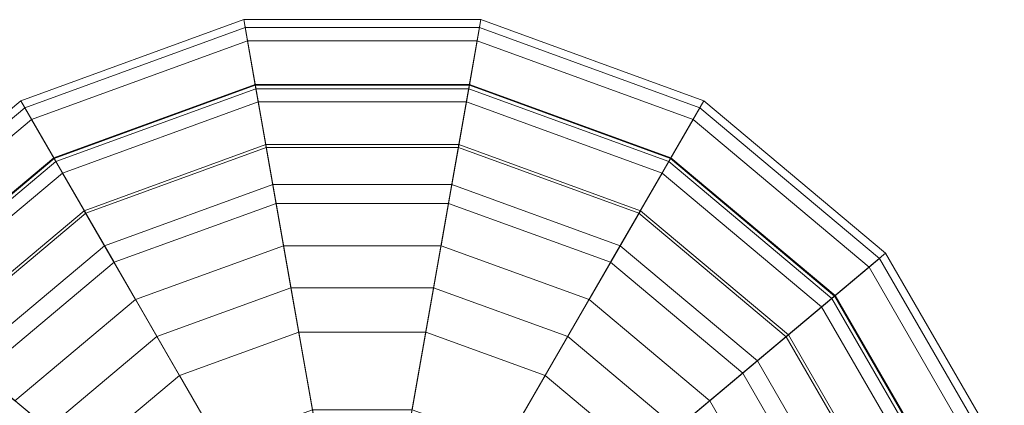
# Model space of a CAD drawing. Units: inches. Extents: x 375 to 1122, y 27 to 1069.
# Tile 23 of 155: x 718.584 to 720.536, y 273.809 to 274.574. Entities that reach past the tile are written whole.
import ezdxf

# ---------------------------------------------------------------- set-up
doc = ezdxf.new("R2010")
doc.units = ezdxf.units.IN
doc.layers.add('Furniture', color=30, linetype='Continuous', lineweight=18)

# ---------------------------------------------------------------- blocks, each defined once
blk = doc.blocks.new('A$C403C54AD')
for points in [[(1.816094, 0.886635, -0.028594), (1.814977, 0.889704, -0.031825), (1.804793, 0.883824, -0.031825), (1.806892, 0.881322, -0.028594)], [(1.814977, 0.889704, -0.031825), (1.826559, 0.857884, -0.028747), (1.826559, 0.857884, -0.028747), (1.804793, 0.883824, -0.031825)], [(1.816108, 0.886597, 0.131159), (1.815114, 0.889329, 0.117935), (1.805049, 0.883518, 0.117935), (1.806918, 0.881291, 0.131159)], [(1.815114, 0.889329, 0.117935), (1.815345, 0.888695, 0.089693), (1.805483, 0.883001, 0.089693), (1.805049, 0.883518, 0.117935)], [(1.815345, 0.888695, 0.089693), (1.817179, 0.883654, 0.071684), (1.808931, 0.878892, 0.071684), (1.805483, 0.883001, 0.089693)], [(1.821697, 0.871241, -0.02532), (1.816094, 0.886635, -0.028594), (1.806892, 0.881322, -0.028594), (1.817422, 0.868773, -0.02532)], [(1.817817, 0.881902, 0.140564), (1.816108, 0.886597, 0.131159), (1.806918, 0.881291, 0.131159), (1.81013, 0.877464, 0.140564)], [(1.816169, 0.886431, 0.117718), (1.81713, 0.88379, 0.130354), (1.808838, 0.879003, 0.130354), (1.807032, 0.881156, 0.117718)], [(1.816394, 0.885812, 0.090178), (1.816169, 0.886431, 0.117718), (1.807032, 0.881156, 0.117718), (1.807455, 0.880651, 0.090178)], [(1.818141, 0.881013, 0.073031), (1.816394, 0.885812, 0.090178), (1.807455, 0.880651, 0.090178), (1.810738, 0.876739, 0.073031)], [(1.806892, 0.881322, -0.028594), (1.804793, 0.883824, -0.031825), (1.797233, 0.874815, -0.031825), (1.800062, 0.873182, -0.028594)], [(1.804793, 0.883824, -0.031825), (1.826559, 0.857884, -0.028747), (1.826559, 0.857884, -0.028747), (1.797233, 0.874815, -0.031825)], [(1.806918, 0.881291, 0.131159), (1.805049, 0.883518, 0.117935), (1.797579, 0.874616, 0.117935), (1.800097, 0.873162, 0.131159)], [(1.805049, 0.883518, 0.117935), (1.805483, 0.883001, 0.089693), (1.798163, 0.874278, 0.089693), (1.797579, 0.874616, 0.117935)], [(1.81713, 0.88379, 0.130354), (1.81887, 0.879009, 0.140564), (1.812108, 0.875106, 0.140564), (1.808838, 0.879003, 0.130354)], [(1.817179, 0.883654, 0.071684), (1.819596, 0.877014, 0.061451), (1.813473, 0.873479, 0.061451), (1.808931, 0.878892, 0.071684)], [(1.805483, 0.883001, 0.089693), (1.808931, 0.878892, 0.071684), (1.802809, 0.871596, 0.071684), (1.798163, 0.874278, 0.089693)], [(1.81887, 0.879009, 0.140564), (1.817817, 0.881902, 0.140564), (1.81013, 0.877464, 0.140564), (1.812108, 0.875106, 0.140564)], [(1.817422, 0.868773, -0.02532), (1.806892, 0.881322, -0.028594), (1.800062, 0.873182, -0.028594), (1.814249, 0.864991, -0.02532)], [(1.81013, 0.877464, 0.140564), (1.806918, 0.881291, 0.131159), (1.800097, 0.873162, 0.131159), (1.804424, 0.870664, 0.140564)], [(1.807032, 0.881156, 0.117718), (1.808838, 0.879003, 0.130354), (1.802683, 0.871669, 0.130354), (1.80025, 0.873073, 0.117718)], [(1.807455, 0.880651, 0.090178), (1.807032, 0.881156, 0.117718), (1.80025, 0.873073, 0.117718), (1.80082, 0.872744, 0.090178)], [(1.820359, 0.874918, 0.063639), (1.818141, 0.881013, 0.073031), (1.810738, 0.876739, 0.073031), (1.814907, 0.87177, 0.063639)], [(1.810738, 0.876739, 0.073031), (1.807455, 0.880651, 0.090178), (1.80082, 0.872744, 0.090178), (1.805243, 0.87019, 0.073031)], [(1.808838, 0.879003, 0.130354), (1.812108, 0.875106, 0.140564), (1.80709, 0.869125, 0.140564), (1.802683, 0.871669, 0.130354)], [(1.808931, 0.878892, 0.071684), (1.813473, 0.873479, 0.061451), (1.808929, 0.868063, 0.061451), (1.802809, 0.871596, 0.071684)], [(1.812108, 0.875106, 0.140564), (1.81013, 0.877464, 0.140564), (1.804424, 0.870664, 0.140564), (1.80709, 0.869125, 0.140564)], [(1.814907, 0.87177, 0.063639), (1.810738, 0.876739, 0.073031), (1.805243, 0.87019, 0.073031), (1.81086, 0.866948, 0.063639)], [(1.800062, 0.873182, -0.028594), (1.797233, 0.874815, -0.031825), (1.793211, 0.863764, -0.031825), (1.796427, 0.863197, -0.028594)], [(1.797233, 0.874815, -0.031825), (1.826559, 0.857884, -0.028747), (1.826559, 0.857884, -0.028747), (1.793211, 0.863764, -0.031825)], [(1.800097, 0.873162, 0.131159), (1.797579, 0.874616, 0.117935), (1.793604, 0.863695, 0.117935), (1.796467, 0.86319, 0.131159)], [(1.797579, 0.874616, 0.117935), (1.798163, 0.874278, 0.089693), (1.794269, 0.863578, 0.089693), (1.793604, 0.863695, 0.117935)], [(1.798163, 0.874278, 0.089693), (1.802809, 0.871596, 0.071684), (1.799552, 0.862646, 0.071684), (1.794269, 0.863578, 0.089693)], [(1.814249, 0.864991, -0.02532), (1.800062, 0.873182, -0.028594), (1.796427, 0.863197, -0.028594), (1.812561, 0.860352, -0.02532)], [(1.804424, 0.870664, 0.140564), (1.800097, 0.873162, 0.131159), (1.796467, 0.86319, 0.131159), (1.801388, 0.862322, 0.140564)], [(1.813473, 0.873479, 0.061451), (1.820055, 0.865635, 0.054084), (1.817796, 0.862943, 0.054084), (1.808929, 0.868063, 0.061451)], [(1.80025, 0.873073, 0.117718), (1.802683, 0.871669, 0.130354), (1.799409, 0.862671, 0.130354), (1.796642, 0.863159, 0.117718)], [(1.80082, 0.872744, 0.090178), (1.80025, 0.873073, 0.117718), (1.796642, 0.863159, 0.117718), (1.79729, 0.863045, 0.090178)], [(1.805243, 0.87019, 0.073031), (1.80082, 0.872744, 0.090178), (1.79729, 0.863045, 0.090178), (1.80232, 0.862158, 0.073031)], [(1.802683, 0.871669, 0.130354), (1.80709, 0.869125, 0.140564), (1.804419, 0.861788, 0.140564), (1.799409, 0.862671, 0.130354)], [(1.820835, 0.864705, 0.057003), (1.814907, 0.87177, 0.063639), (1.81086, 0.866948, 0.063639), (1.818848, 0.862336, 0.057003)], [(1.802809, 0.871596, 0.071684), (1.808929, 0.868063, 0.061451), (1.806511, 0.861419, 0.061451), (1.799552, 0.862646, 0.071684)], [(1.80709, 0.869125, 0.140564), (1.804424, 0.870664, 0.140564), (1.801388, 0.862322, 0.140564), (1.804419, 0.861788, 0.140564)], [(1.81086, 0.866948, 0.063639), (1.805243, 0.87019, 0.073031), (1.80232, 0.862158, 0.073031), (1.808707, 0.861032, 0.063639)], [(1.808929, 0.868063, 0.061451), (1.817796, 0.862943, 0.054084), (1.816594, 0.859641, 0.054084), (1.806511, 0.861419, 0.061451)], [(1.818848, 0.862336, 0.057003), (1.81086, 0.866948, 0.063639), (1.808707, 0.861032, 0.063639), (1.81779, 0.85943, 0.057003)], [(1.796427, 0.863197, -0.028594), (1.793211, 0.863764, -0.031825), (1.793211, 0.852004, -0.031825), (1.796427, 0.852571, -0.028594)], [(1.793211, 0.863764, -0.031825), (1.826559, 0.857884, -0.028747), (1.826559, 0.857884, -0.028747), (1.793211, 0.852004, -0.031825)], [(1.796467, 0.86319, 0.131159), (1.793604, 0.863695, 0.117935), (1.793604, 0.852073, 0.117935), (1.796467, 0.852578, 0.131159)], [(1.793604, 0.863695, 0.117935), (1.794269, 0.863578, 0.089693), (1.794269, 0.85219, 0.089693), (1.793604, 0.852073, 0.117935)], [(1.794269, 0.863578, 0.089693), (1.799552, 0.862646, 0.071684), (1.799552, 0.853122, 0.071684), (1.794269, 0.85219, 0.089693)], [(1.812561, 0.860352, -0.02532), (1.796427, 0.863197, -0.028594), (1.796427, 0.852571, -0.028594), (1.812561, 0.855416, -0.02532)], [(1.801388, 0.862322, 0.140564), (1.796467, 0.86319, 0.131159), (1.796467, 0.852578, 0.131159), (1.801388, 0.853446, 0.140564)], [(1.796642, 0.863159, 0.117718), (1.799409, 0.862671, 0.130354), (1.799409, 0.853097, 0.130354), (1.796642, 0.852609, 0.117718)], [(1.79729, 0.863045, 0.090178), (1.796642, 0.863159, 0.117718), (1.796642, 0.852609, 0.117718), (1.79729, 0.852723, 0.090178)], [(1.80232, 0.862158, 0.073031), (1.79729, 0.863045, 0.090178), (1.79729, 0.852723, 0.090178), (1.80232, 0.85361, 0.073031)], [(1.799409, 0.862671, 0.130354), (1.804419, 0.861788, 0.140564), (1.804419, 0.85398, 0.140564), (1.799409, 0.853097, 0.130354)], [(1.799552, 0.862646, 0.071684), (1.806511, 0.861419, 0.061451), (1.806511, 0.854349, 0.061451), (1.799552, 0.853122, 0.071684)], [(1.804419, 0.861788, 0.140564), (1.801388, 0.862322, 0.140564), (1.801388, 0.853446, 0.140564), (1.804419, 0.85398, 0.140564)], [(1.808707, 0.861032, 0.063639), (1.80232, 0.862158, 0.073031), (1.80232, 0.85361, 0.073031), (1.808707, 0.854736, 0.063639)], [(1.806511, 0.861419, 0.061451), (1.816594, 0.859641, 0.054084), (1.816594, 0.856127, 0.054084), (1.806511, 0.854349, 0.061451)], [(1.81779, 0.85943, 0.057003), (1.808707, 0.861032, 0.063639), (1.808707, 0.854736, 0.063639), (1.81779, 0.856338, 0.057003)], [(1.793211, 0.852004, -0.031825), (1.826559, 0.857884, -0.028747), (1.826559, 0.857884, -0.028747), (1.797233, 0.840953, -0.031825)], [(1.797233, 0.840953, -0.031825), (1.826559, 0.857884, -0.028747), (1.826559, 0.857884, -0.028747), (1.804793, 0.831944, -0.031825)], [(1.804793, 0.831944, -0.031825), (1.826559, 0.857884, -0.028747), (1.826559, 0.857884, -0.028747), (1.814977, 0.826064, -0.031825)], [(1.806511, 0.854349, 0.061451), (1.816594, 0.856127, 0.054084), (1.817796, 0.852825, 0.054084), (1.808929, 0.847705, 0.061451)], [(1.81779, 0.856338, 0.057003), (1.808707, 0.854736, 0.063639), (1.81086, 0.84882, 0.063639), (1.818848, 0.853432, 0.057003)], [(1.812561, 0.855416, -0.02532), (1.796427, 0.852571, -0.028594), (1.800062, 0.842586, -0.028594), (1.814249, 0.850777, -0.02532)], [(1.808707, 0.854736, 0.063639), (1.80232, 0.85361, 0.073031), (1.805243, 0.845577, 0.073031), (1.81086, 0.84882, 0.063639)], [(1.799552, 0.853122, 0.071684), (1.806511, 0.854349, 0.061451), (1.808929, 0.847705, 0.061451), (1.802809, 0.844172, 0.071684)], [(1.80232, 0.85361, 0.073031), (1.79729, 0.852723, 0.090178), (1.80082, 0.843024, 0.090178), (1.805243, 0.845577, 0.073031)], [(1.799409, 0.853097, 0.130354), (1.804419, 0.85398, 0.140564), (1.80709, 0.846643, 0.140564), (1.802683, 0.844099, 0.130354)], [(1.804419, 0.85398, 0.140564), (1.801388, 0.853446, 0.140564), (1.804424, 0.845104, 0.140564), (1.80709, 0.846643, 0.140564)], [(1.794269, 0.85219, 0.089693), (1.799552, 0.853122, 0.071684), (1.802809, 0.844172, 0.071684), (1.798163, 0.84149, 0.089693)], [(1.801388, 0.853446, 0.140564), (1.796467, 0.852578, 0.131159), (1.800097, 0.842606, 0.131159), (1.804424, 0.845104, 0.140564)], [(1.796642, 0.852609, 0.117718), (1.799409, 0.853097, 0.130354), (1.802683, 0.844099, 0.130354), (1.80025, 0.842695, 0.117718)], [(1.818848, 0.853432, 0.057003), (1.81086, 0.84882, 0.063639), (1.814907, 0.843998, 0.063639), (1.820835, 0.851063, 0.057003)], [(1.79729, 0.852723, 0.090178), (1.796642, 0.852609, 0.117718), (1.80025, 0.842695, 0.117718), (1.80082, 0.843024, 0.090178)], [(1.808929, 0.847705, 0.061451), (1.817796, 0.852825, 0.054084), (1.820055, 0.850133, 0.054084), (1.813473, 0.842289, 0.061451)], [(1.796427, 0.852571, -0.028594), (1.793211, 0.852004, -0.031825), (1.797233, 0.840953, -0.031825), (1.800062, 0.842586, -0.028594)], [(1.796467, 0.852578, 0.131159), (1.793604, 0.852073, 0.117935), (1.797579, 0.841152, 0.117935), (1.800097, 0.842606, 0.131159)], [(1.793604, 0.852073, 0.117935), (1.794269, 0.85219, 0.089693), (1.798163, 0.84149, 0.089693), (1.797579, 0.841152, 0.117935)], [(1.814249, 0.850777, -0.02532), (1.800062, 0.842586, -0.028594), (1.806892, 0.834446, -0.028594), (1.817422, 0.846995, -0.02532)], [(1.81086, 0.84882, 0.063639), (1.805243, 0.845577, 0.073031), (1.810738, 0.839029, 0.073031), (1.814907, 0.843998, 0.063639)], [(1.802809, 0.844172, 0.071684), (1.808929, 0.847705, 0.061451), (1.813473, 0.842289, 0.061451), (1.808931, 0.836876, 0.071684)], [(1.817422, 0.846995, -0.02532), (1.806892, 0.834446, -0.028594), (1.816094, 0.829133, -0.028594), (1.821697, 0.844527, -0.02532)], [(1.802683, 0.844099, 0.130354), (1.80709, 0.846643, 0.140564), (1.812108, 0.840662, 0.140564), (1.808838, 0.836765, 0.130354)], [(1.80709, 0.846643, 0.140564), (1.804424, 0.845104, 0.140564), (1.81013, 0.838304, 0.140564), (1.812108, 0.840662, 0.140564)], [(1.805243, 0.845577, 0.073031), (1.80082, 0.843024, 0.090178), (1.807455, 0.835117, 0.090178), (1.810738, 0.839029, 0.073031)], [(1.804424, 0.845104, 0.140564), (1.800097, 0.842606, 0.131159), (1.806918, 0.834477, 0.131159), (1.81013, 0.838304, 0.140564)], [(1.798163, 0.84149, 0.089693), (1.802809, 0.844172, 0.071684), (1.808931, 0.836876, 0.071684), (1.805483, 0.832767, 0.089693)], [(1.80025, 0.842695, 0.117718), (1.802683, 0.844099, 0.130354), (1.808838, 0.836765, 0.130354), (1.807032, 0.834612, 0.117718)], [(1.814907, 0.843998, 0.063639), (1.810738, 0.839029, 0.073031), (1.818141, 0.834755, 0.073031), (1.820359, 0.84085, 0.063639)], [(1.80082, 0.843024, 0.090178), (1.80025, 0.842695, 0.117718), (1.807032, 0.834612, 0.117718), (1.807455, 0.835117, 0.090178)], [(1.800062, 0.842586, -0.028594), (1.797233, 0.840953, -0.031825), (1.804793, 0.831944, -0.031825), (1.806892, 0.834446, -0.028594)], [(1.800097, 0.842606, 0.131159), (1.797579, 0.841152, 0.117935), (1.805049, 0.83225, 0.117935), (1.806918, 0.834477, 0.131159)], [(1.808931, 0.836876, 0.071684), (1.813473, 0.842289, 0.061451), (1.819596, 0.838754, 0.061451), (1.817179, 0.832114, 0.071684)], [(1.797579, 0.841152, 0.117935), (1.798163, 0.84149, 0.089693), (1.805483, 0.832767, 0.089693), (1.805049, 0.83225, 0.117935)]]:
    blk.add_3dface(points)

msp = doc.modelspace()

# ---------------------------------------------------------------- block references
at = {"layer": 'Furniture', "xscale": 39.9918517141215, "yscale": 39.9918517141215, "zscale": 39.9918517141215, "rotation": 270}
msp.add_blockref('A$C403C54AD', (684.9549, 346.2875, 0.024), dxfattribs=at)

doc.saveas('drawing.dxf')
